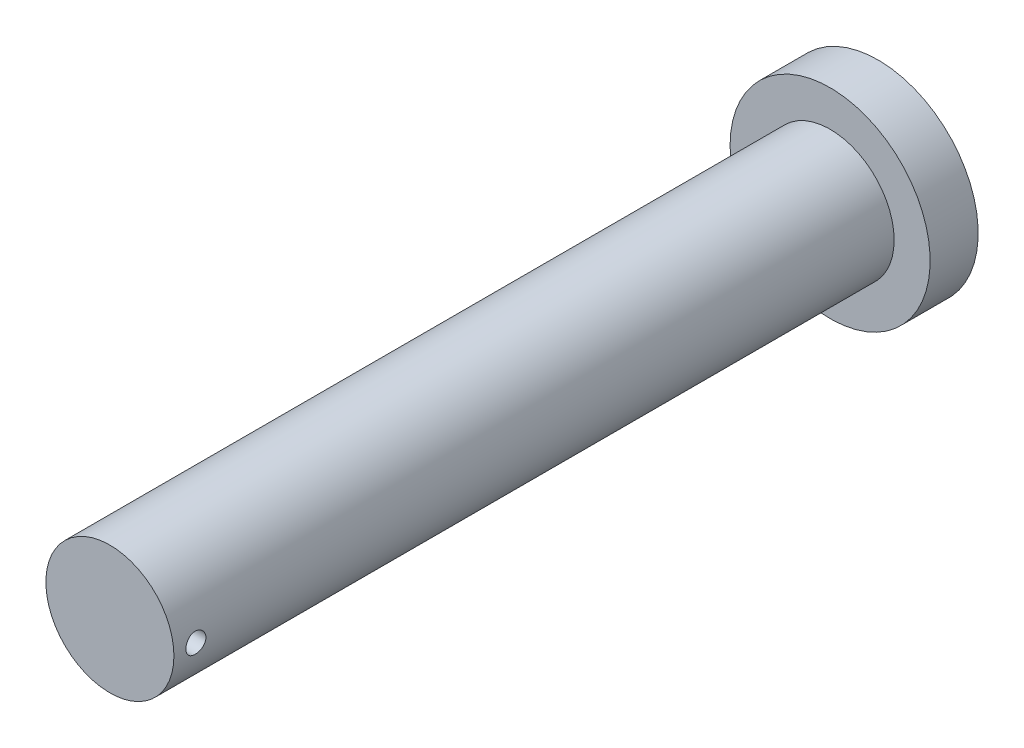
from build123d import *

# Parameters (mm, degrees)
SHANK_PROFILE_32_R     = 16
SHANK_32X180_DEPTH     = 180
HEAD_PROFILE_50_R      = 25
HEAD_50X12_DEPTH       = 12
CROSS_HOLE_PROFILE_5_R = 2.5
CROSS_HOLE_5_DEPTH     = 75


with BuildPart() as part:
    # Shank Profile Ø32 → Shank Ø32x180 (new body)
    with BuildSketch(Plane.XY):
        with Locations(Location((0, 0, 0), (0, 0, 180))):
            Circle(SHANK_PROFILE_32_R)
    extrude(amount=SHANK_32X180_DEPTH)

    # Head Profile Ø50 → Head Ø50x12 (add)
    with BuildSketch(Plane(origin=(0, 0, 0), x_dir=(-1, 0, 0), z_dir=(0, 0, -1))):
        Circle(HEAD_PROFILE_50_R)
    extrude(amount=HEAD_50X12_DEPTH)

    # Cross Hole Profile Ø5 → Cross Hole Ø5 (cut, symmetric)
    with BuildSketch(Plane(origin=(0, 0, 0), x_dir=(0, 0, -1), z_dir=(1, 0, 0))):
        with Locations(Location((-174.5, 0, 0), (0, 0, 180))):
            Circle(CROSS_HOLE_PROFILE_5_R)
    extrude(amount=CROSS_HOLE_5_DEPTH, both=True, mode=Mode.SUBTRACT)


solid = part.part
